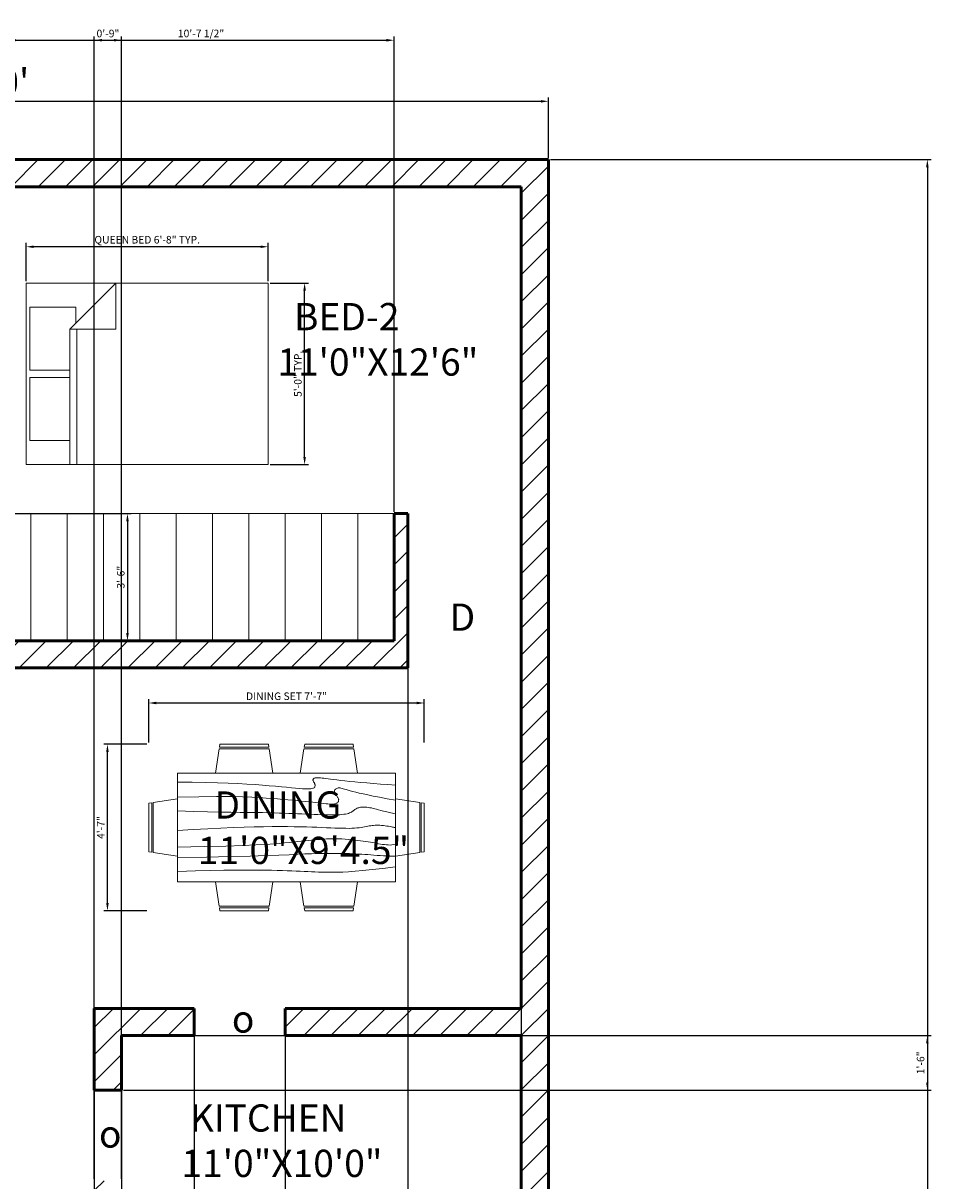
# Model space of a CAD drawing. Units: inches. Extents: x 2758 to 3288, y 1211 to 2050.
# Tile 4 of 4: x 2988 to 3288, y 1667 to 2050. Entities that reach past the tile are written whole.
import ezdxf

# ---------------------------------------------------------------- set-up
doc = ezdxf.new("R2010")
doc.units = ezdxf.units.IN
for name, color, linetype, lineweight in [('A-ANNO-DIMS', 2, 'Continuous', 18), ('A-AREA-IDEN', 7, 'Continuous', 25), ('A-FURN', 8, 'Continuous', 18), ('A-WALL', 7, 'Continuous', 50)]:
    doc.layers.add(name, color=color, linetype=linetype, lineweight=lineweight)
for name, color, linetype, lineweight, true_color in [('A-ANNO-TEXT', 244, 'Continuous', 18, 0x991b1e), ('A-FLOR-CASE', 244, 'Continuous', 18, 0x991b1e), ('A-WALL-PATT', 244, 'Continuous', 13, 0x991b1e)]:
    doc.layers.add(name, color=color, linetype=linetype, lineweight=lineweight, true_color=true_color)
doc.styles.get("Standard").update_dxf_attribs({"font": 'arial.ttf'})
doc.dimstyles.new('ISO-25', dxfattribs={"dimtxt": 2.5, "dimasz": 2.5, "dimexe": 1.25, "dimexo": 0.625, "dimtad": 1, "dimlunit": 3, "dimtxsty": 'Standard', "dimcen": 2.5, "dimadec": 0, "dimazin": 0, "dimtfac": 1, "dimtmove": 0, "dimatfit": 3, "dimfxl": 1, "dimarcsym": 0})

# ---------------------------------------------------------------- blocks, each defined once
blk = doc.blocks.new('Dining Set - 36 x 72 in.')
for p, q in [((-22, 27.5), (-22.1562, 26.50042)), ((-22, 27.5), (-6, 27.5)), ((-5.8437, 26.49966), (-6, 27.5)), ((6, 27.5), (5.8438, 26.50042)), ((6, 27.5), (22, 27.5)), ((22.1563, 26.49966), (22, 27.5)), ((-22.2343, 26.00059), (-23.4847, 17.99762)), ((-22.2304, 26), (-5.7608, 26)), ((-5.8416, 26.5), (-22.1534, 26.5)), ((-4.5152, 17.99762), (-5.7655, 25.99926)), ((5.7657, 26.00059), (4.5153, 17.99762)), ((5.7696, 26), (22.2392, 26)), ((22.1584, 26.5), (5.8466, 26.5)), ((23.4848, 17.99762), (22.2345, 25.99926)), ((36, 18), (-36, 18)), ((-36, 18), (-36, -18)), ((36, -18), (36, 18)), ((-45.5, 8), (-44.5004, 8.15617)), ((-45.5, 8), (-45.5, -8)), ((-44.5, -8.15843), (-44.5, 8.15338)), ((-44.0006, 8.23428), (-35.9976, 9.48474)), ((-44, 8.23041), (-44, -8.23915)), ((44.0006, 8.23428), (35.9976, 9.48474)), ((44, 8.23041), (44, -8.23915)), ((44.5, -8.15843), (44.5, 8.15338)), ((45.5, 8), (44.5005, 8.15617)), ((45.5, 8), (45.5, -8)), ((-44.4997, -8.15631), (-45.5, -8)), ((-35.9976, -9.48476), (-43.9993, -8.2345)), ((35.9976, -9.48476), (43.9993, -8.2345)), ((44.4997, -8.15631), (45.5, -8)), ((-36, -18), (36, -18)), ((-22.2343, -26.0006), (-23.4847, -17.99762)), ((-4.5152, -17.99762), (-5.7655, -25.99928)), ((5.7657, -26.0006), (4.5153, -17.99762)), ((23.4848, -17.99762), (22.2345, -25.99928)), ((-22.2304, -26), (-5.7608, -26)), ((-22, -27.5), (-22.1562, -26.50044)), ((-5.8416, -26.5), (-22.1534, -26.5)), ((-5.8437, -26.49967), (-6, -27.5)), ((5.7696, -26), (22.2392, -26)), ((6, -27.5), (5.8438, -26.50044)), ((22.1584, -26.5), (5.8466, -26.5)), ((22.1563, -26.49967), (22, -27.5)), ((-22, -27.5), (-6, -27.5)), ((6, -27.5), (22, -27.5))]:
    blk.add_line(p, q)
for points in [[(-36, 15), (-31.1772, 14.97754), (-26.8079, 14.91406), (-22.8538, 14.81543), (-19.276, 14.6875), (-16.0362, 14.53613), (-13.0957, 14.36718), (-10.4159, 14.18652), (-7.9583, 14), (-5.6904, 13.81315), (-3.6035, 13.63021), (-1.6954, 13.45508), (0.0365, 13.29166), (1.5945, 13.14388), (2.9811, 13.01562), (4.1988, 12.9108), (5.25, 12.83333), (6.1393, 12.78613), (6.8802, 12.76823), (7.4883, 12.77767), (7.9792, 12.8125), (8.3685, 12.87077), (8.6719, 12.95052), (8.9049, 13.0498), (9.0833, 13.16666), (9.2205, 13.29899), (9.3216, 13.44401), (9.3895, 13.59879), (9.4271, 13.76041), (9.4373, 13.92594), (9.4232, 14.09245), (9.3875, 14.257), (9.3333, 14.41666), (9.2638, 14.56917), (9.1836, 14.71484), (9.0975, 14.85465), (9.0104, 14.98958), (8.9272, 15.1206), (8.8529, 15.2487), (8.7922, 15.37483), (8.75, 15.5), (8.7305, 15.62467), (8.7344, 15.74739), (8.7617, 15.86621), (8.8125, 15.97916), (8.8867, 16.08431), (8.9844, 16.17968), (9.1055, 16.26334), (9.25, 16.33333), (9.4189, 16.38802), (9.6172, 16.42708), (9.8506, 16.45052), (10.125, 16.45833), (10.4463, 16.45052), (10.8203, 16.42708), (11.2529, 16.38802), (11.75, 16.33333), (12.3184, 16.26318), (12.9694, 16.17838), (13.7151, 16.07991), (14.5677, 15.96875), (15.5395, 15.84586), (16.6426, 15.71224), (17.8893, 15.56884), (19.2917, 15.41666), (20.859, 15.25667), (22.5879, 15.08984), (24.4721, 14.91715), (26.5052, 14.73958), (28.6809, 14.5581), (30.9929, 14.3737), (33.4347, 14.18733), (36, 14)], [(-36, 10), (-28.9766, 10.14274), (-23.1725, 10.20442), (-18.4241, 10.19775), (-14.5677, 10.13541), (-11.4399, 10.03011), (-8.877, 9.89453), (-6.7154, 9.74137), (-4.7917, 9.58333), (-2.9698, 9.43082), (-1.2246, 9.28515), (0.4415, 9.14534), (2.026, 9.01041), (3.5266, 8.87939), (4.9408, 8.7513), (6.266, 8.62516), (7.5, 8.5), (8.6411, 8.37549), (9.6914, 8.2539), (10.6538, 8.13818), (11.5312, 8.03125), (12.3267, 7.93603), (13.043, 7.85547), (13.6831, 7.79248), (14.25, 7.75), (14.7471, 7.7303), (15.1797, 7.73307), (15.5537, 7.75732), (15.875, 7.80208), (16.1494, 7.86637), (16.3828, 7.94922), (16.5811, 8.04964), (16.75, 8.16666), (16.8944, 8.29915), (17.0143, 8.44531), (17.1089, 8.60319), (17.1771, 8.77083), (17.218, 8.94629), (17.2305, 9.1276), (17.2137, 9.31282), (17.1667, 9.5), (17.0895, 9.6875), (16.987, 9.875), (16.8649, 10.0625), (16.7292, 10.25), (16.5856, 10.4375), (16.4401, 10.625), (16.2985, 10.8125), (16.1667, 11), (16.05, 11.18733), (15.9518, 11.3737), (15.8752, 11.5581), (15.8229, 11.73958), (15.798, 11.91715), (15.8034, 12.08984), (15.842, 12.25667), (15.9167, 12.41666), (16.0295, 12.56836), (16.1784, 12.70833), (16.3605, 12.83268), (16.5729, 12.9375), (16.8127, 13.01888), (17.0768, 13.07291), (17.3625, 13.0957), (17.6667, 13.08333), (17.9894, 13.03312), (18.3418, 12.94726), (18.7382, 12.82918), (19.1927, 12.68229), (19.7195, 12.51001), (20.3327, 12.31575), (21.0465, 12.10294), (21.875, 11.875), (22.8357, 11.63354), (23.959, 11.37304), (25.2786, 11.08618), (26.8282, 10.76562), (28.6414, 10.40405), (30.752, 9.99414), (33.1936, 9.52856), (36, 9)], [(-36, 5.5), (-30.7157, 5.3348), (-26.069, 5.20963), (-21.9946, 5.11767), (-18.4271, 5.05208), (-15.3009, 5.00602), (-12.5508, 4.97265), (-10.1112, 4.94515), (-7.9167, 4.91666), (-5.909, 4.88167), (-4.0586, 4.83984), (-2.3429, 4.79215), (-0.7396, 4.73958), (0.7739, 4.6831), (2.22, 4.6237), (3.6213, 4.56233), (5, 4.5), (6.373, 4.43782), (7.7344, 4.3776), (9.0723, 4.32129), (10.375, 4.27083), (11.6309, 4.22819), (12.8281, 4.19531), (13.9551, 4.17415), (15, 4.16666), (15.954, 4.17448), (16.819, 4.19791), (17.6001, 4.23698), (18.3021, 4.29166), (18.9299, 4.36198), (19.4883, 4.44791), (19.9823, 4.54948), (20.4167, 4.66666), (20.7969, 4.79899), (21.1302, 4.94401), (21.4245, 5.09879), (21.6875, 5.26041), (21.9271, 5.42594), (22.1511, 5.59245), (22.3672, 5.757), (22.5834, 5.91666), (22.8065, 6.06868), (23.0404, 6.21093), (23.2879, 6.34147), (23.5521, 6.45833), (23.8358, 6.55957), (24.142, 6.64323), (24.4735, 6.70735), (24.8334, 6.75), (25.2235, 6.76969), (25.642, 6.76692), (26.0858, 6.74267), (26.5521, 6.69791), (27.0379, 6.63362), (27.5404, 6.55078), (28.0565, 6.45036), (28.5834, 6.33333), (29.1242, 6.19987), (29.7071, 6.04687), (30.3661, 5.87044), (31.1354, 5.66666), (32.0493, 5.43164), (33.142, 5.16146), (34.4475, 4.85221), (36, 4.5)], [(-36, -1), (-30.7915, -0.6591), (-26.0195, -0.38216), (-21.6519, -0.16284), (-17.6563, 0.00521), (-14.0005, 0.12833), (-10.6523, 0.21289), (-7.5796, 0.26522), (-4.75, 0.29166), (-2.134, 0.29793), (0.2878, 0.28711), (2.5317, 0.26163), (4.6146, 0.22396), (6.5529, 0.17651), (8.3633, 0.12174), (10.0623, 0.06209), (11.6667, 0), (13.1899, -0.06201), (14.6341, -0.1211), (15.9982, -0.17432), (17.2813, -0.21875), (18.4823, -0.25147), (19.6003, -0.26953), (20.6343, -0.27002), (21.5834, -0.25), (22.4481, -0.20768), (23.2357, -0.14584), (23.9549, -0.06836), (24.6146, 0.02083), (25.2235, 0.11784), (25.7904, 0.21875), (26.3241, 0.31966), (26.8334, 0.41666), (27.3265, 0.50618), (27.8099, 0.58593), (28.2894, 0.65397), (28.7709, 0.70833), (29.2601, 0.74707), (29.763, 0.76823), (30.2855, 0.76985), (30.8334, 0.75), (31.4088, 0.70784), (31.9994, 0.64713), (32.589, 0.57275), (33.1615, 0.48958), (33.7008, 0.4025), (34.1908, 0.3164), (34.6153, 0.23616), (34.9584, 0.16666), (35.2099, 0.11165), (35.3848, 0.07031), (35.504, 0.04069), (35.5886, 0.02083), (35.6594, 0.00879), (35.7377, 0.0026), (35.8442, 0.00032), (36, 0)], [(-36, -6.5), (-27.1843, -6.31267), (-20.084, -6.1263), (-14.469, -5.9419), (-10.1094, -5.76042), (-6.7752, -5.58285), (-4.2363, -5.41016), (-2.2629, -5.24333), (-0.625, -5.08334), (0.8708, -4.93099), (2.2715, -4.78646), (3.5872, -4.64974), (4.8281, -4.52084), (6.0046, -4.39974), (7.127, -4.28646), (8.2053, -4.18099), (9.25, -4.08334), (10.2705, -3.99382), (11.2734, -3.91407), (12.2647, -3.84603), (13.25, -3.79167), (14.2354, -3.75293), (15.2266, -3.73177), (16.2295, -3.73015), (17.25, -3.75), (18.2912, -3.79248), (19.3451, -3.85547), (20.4009, -3.93604), (21.4479, -4.03125), (22.4754, -4.13819), (23.4727, -4.25391), (24.4289, -4.37549), (25.3334, -4.5), (26.1785, -4.62492), (26.9694, -4.74935), (27.7145, -4.87281), (28.4219, -4.99479), (29.1, -5.11483), (29.7572, -5.23242), (30.4016, -5.34709), (31.0417, -5.45834), (31.6837, -5.56437), (32.3262, -5.65821), (32.9658, -5.73153), (33.599, -5.77604), (34.2224, -5.78345), (34.8327, -5.74545), (35.4264, -5.65373), (36, -5.5)], [(-36, -10), (-26.4022, -9.81299), (-18.4675, -9.62891), (-11.9839, -9.45069), (-6.7396, -9.28125), (-2.5226, -9.12354), (0.8789, -8.98047), (3.6769, -8.85498), (6.0833, -8.75), (8.2767, -8.66765), (10.3021, -8.60677), (12.1712, -8.56543), (13.8958, -8.54167), (15.4876, -8.53353), (16.9583, -8.53907), (18.3197, -8.55632), (19.5834, -8.58334), (20.7616, -8.61841), (21.8685, -8.66081), (22.9188, -8.71004), (23.9271, -8.76563), (24.9081, -8.82707), (25.8763, -8.89388), (26.8465, -8.96558), (27.8334, -9.04167), (28.8474, -9.12118), (29.8828, -9.20117), (30.93, -9.27824), (31.9792, -9.34896), (33.0205, -9.40991), (34.0443, -9.45768), (35.0407, -9.48885), (36, -9.5)], [(-36, -14.5), (-30.0881, -14.33513), (-25.0332, -14.21224), (-20.7312, -14.12647), (-17.0781, -14.07292), (-13.97, -14.04671), (-11.3027, -14.04297), (-8.9724, -14.05681), (-6.875, -14.08334), (-4.9224, -14.11833), (-3.0905, -14.16016), (-1.3709, -14.20785), (0.2448, -14.26042), (1.7647, -14.3169), (3.1973, -14.3763), (4.5507, -14.43767), (5.8333, -14.5), (7.0554, -14.5621), (8.235, -14.62175), (9.3922, -14.67652), (10.5469, -14.72396), (11.7192, -14.76164), (12.929, -14.78711), (14.1965, -14.79794), (15.5417, -14.79167), (16.9933, -14.76424), (18.6152, -14.70508), (20.4804, -14.60197), (22.6615, -14.44271), (25.2312, -14.21509), (28.2624, -13.9069), (31.8277, -13.50594), (36, -13)]]:
    blk.add_lwpolyline(points)
blk = doc.blocks.new('Bed - Queen')
for p, q in [((0, -80.00003), (0, 0)), ((0, 0), (59.99999, 0)), ((59.99999, 0), (59.99999, -80.00003)), ((7.99999, -1.2), (28.79998, -1.2)), ((7.99999, -14.4), (7.99999, -1.2)), ((28.79998, -1.2), (28.79998, -14.4)), ((31.19999, -1.2), (51.99999, -1.2)), ((31.19999, -14.4), (31.19999, -1.2)), ((51.99999, -1.2), (51.99999, -16.4)), ((0, -14.4), (44.8, -14.4)), ((59.99999, -29.6), (44.8, -14.4)), ((44.8, -14.4), (44.8, -29.6)), ((44.8, -16.8), (0, -16.8)), ((51.99999, -16.4), (46.79936, -16.4)), ((44.8, -29.6), (59.99999, -29.6)), ((59.99999, -80.00003), (0, -80.00003))]:
    blk.add_line(p, q)
blk = doc.blocks.new('*D6')
at = {"layer": 'A-ANNO-DIMS', "color": 0, "lineweight": -2, "transparency": 16777216}
for p, q in [((2801.14, 2005.44), (2801.14, 2025.32)), ((2803.64, 2024.07), (3158.64, 2024.07)), ((3161.14, 2005.44), (3161.14, 2025.32))]:
    blk.add_line(p, q, dxfattribs=at)
at = {"layer": 'A-ANNO-DIMS', "color": 0, "transparency": 16777216}
for points in [[(2803.64, 2024.49), (2803.64, 2023.65), (2801.14, 2024.07)], [(3158.64, 2024.49), (3158.64, 2023.65), (3161.14, 2024.07)]]:
    blk.add_solid(points, dxfattribs=at)
at = {"layer": 'Defpoints', "color": 0, "transparency": 16777216}
for p in [(3161.14, 2024.07), (2801.14, 2004.81), (3161.14, 2004.81)]:
    blk.add_point(p, dxfattribs=at)
at = {"layer": 'A-ANNO-DIMS', "color": 0, "transparency": 16777216, "insert": (2981.14, 2029.29), "char_height": 9, "attachment_point": 5}
blk.add_mtext("30'", dxfattribs=at)
blk = doc.blocks.new('*D8')
at = {"layer": 'A-ANNO-DIMS', "color": 0, "lineweight": -2, "transparency": 16777216}
for p, q in [((2988.6, 1964.64), (2988.6, 1977.26)), ((3066.1, 1976.01), (2991.1, 1976.01)), ((3068.6, 1964.64), (3068.6, 1977.26))]:
    blk.add_line(p, q, dxfattribs=at)
at = {"layer": 'A-ANNO-DIMS', "color": 0, "transparency": 16777216}
for points in [[(2991.1, 1976.43), (2991.1, 1975.6), (2988.6, 1976.01)], [(3066.1, 1976.43), (3066.1, 1975.6), (3068.6, 1976.01)]]:
    blk.add_solid(points, dxfattribs=at)
at = {"layer": 'Defpoints', "color": 0, "transparency": 16777216}
for p in [(2988.6, 1976.01), (2988.6, 1964.01), (3068.6, 1964.01)]:
    blk.add_point(p, dxfattribs=at)
at = {"layer": 'A-ANNO-DIMS', "color": 0, "transparency": 16777216, "insert": (3028.6, 1978.01), "char_height": 2.5, "attachment_point": 5}
blk.add_mtext('QUEEN BED 6\'-8" TYP.', dxfattribs=at)
blk = doc.blocks.new('*D9')
at = {"layer": 'A-ANNO-DIMS', "color": 0, "lineweight": -2, "transparency": 16777216}
for p, q in [((3069.23, 1964.01), (3081.85, 1964.01)), ((3080.6, 1906.51), (3080.6, 1961.51)), ((3069.23, 1904.01), (3081.85, 1904.01))]:
    blk.add_line(p, q, dxfattribs=at)
at = {"layer": 'A-ANNO-DIMS', "color": 0, "transparency": 16777216}
for points in [[(3080.18, 1961.51), (3081.02, 1961.51), (3080.6, 1964.01)], [(3080.18, 1906.51), (3081.02, 1906.51), (3080.6, 1904.01)]]:
    blk.add_solid(points, dxfattribs=at)
at = {"layer": 'Defpoints', "color": 0, "transparency": 16777216}
for p in [(3068.6, 1964.01), (3080.6, 1964.01), (3068.6, 1904.01)]:
    blk.add_point(p, dxfattribs=at)
at = {"layer": 'A-ANNO-DIMS', "color": 0, "transparency": 16777216, "insert": (3078.7, 1934.01), "char_height": 2.5, "attachment_point": 5, "rotation": 90}
blk.add_mtext('5\'-0" TYP.', dxfattribs=at)
blk = doc.blocks.new('*D12')
at = {"layer": 'A-ANNO-DIMS', "color": 0, "lineweight": -2, "transparency": 16777216}
for p, q in [((3029.13, 1812.2), (3029.13, 1826.48)), ((3031.63, 1825.23), (3117.63, 1825.23)), ((3120.13, 1812.2), (3120.13, 1826.48))]:
    blk.add_line(p, q, dxfattribs=at)
at = {"layer": 'A-ANNO-DIMS', "color": 0, "transparency": 16777216}
for points in [[(3031.63, 1825.65), (3031.63, 1824.81), (3029.13, 1825.23)], [(3117.63, 1825.65), (3117.63, 1824.81), (3120.13, 1825.23)]]:
    blk.add_solid(points, dxfattribs=at)
at = {"layer": 'Defpoints', "color": 0, "transparency": 16777216}
for p in [(3120.13, 1825.23), (3029.13, 1811.58), (3120.13, 1811.58)]:
    blk.add_point(p, dxfattribs=at)
at = {"layer": 'A-ANNO-DIMS', "color": 0, "transparency": 16777216, "insert": (3074.63, 1827.15), "char_height": 2.5, "attachment_point": 5}
blk.add_mtext('DINING SET 7\'-7"', dxfattribs=at)
blk = doc.blocks.new('*D13')
at = {"layer": 'A-ANNO-DIMS', "color": 0, "lineweight": -2, "transparency": 16777216}
for p, q in [((3028.5, 1811.58), (3014.23, 1811.58)), ((3015.48, 1759.08), (3015.48, 1809.08)), ((3028.5, 1756.58), (3014.23, 1756.58))]:
    blk.add_line(p, q, dxfattribs=at)
at = {"layer": 'A-ANNO-DIMS', "color": 0, "transparency": 16777216}
for points in [[(3015.06, 1809.08), (3015.89, 1809.08), (3015.48, 1811.58)], [(3015.06, 1759.08), (3015.89, 1759.08), (3015.48, 1756.58)]]:
    blk.add_solid(points, dxfattribs=at)
at = {"layer": 'Defpoints', "color": 0, "transparency": 16777216}
for p in [(3015.48, 1811.58), (3029.13, 1811.58), (3029.13, 1756.58)]:
    blk.add_point(p, dxfattribs=at)
at = {"layer": 'A-ANNO-DIMS', "color": 0, "transparency": 16777216, "insert": (3013.6, 1784.08), "char_height": 2.5, "attachment_point": 5, "rotation": 90}
blk.add_mtext('4\'-7"', dxfattribs=at)
blk = doc.blocks.new('*D19')
at = {"layer": 'A-ANNO-DIMS', "color": 0, "lineweight": -2, "transparency": 16777216}
for p, q in [((3161.76, 2004.81), (3287.54, 2004.81)), ((3286.29, 2002.31), (3286.29, 1254.6)), ((3247.46, 1252.1), (3287.54, 1252.1))]:
    blk.add_line(p, q, dxfattribs=at)
at = {"layer": 'A-ANNO-DIMS', "color": 0, "transparency": 16777216}
for points in [[(3285.87, 2002.31), (3286.7, 2002.31), (3286.29, 2004.81)], [(3285.87, 1254.6), (3286.7, 1254.6), (3286.29, 1252.1)]]:
    blk.add_solid(points, dxfattribs=at)
at = {"layer": 'Defpoints', "color": 0, "transparency": 16777216}
for p in [(3161.14, 2004.81), (3246.84, 1252.1), (3286.29, 1252.1)]:
    blk.add_point(p, dxfattribs=at)
at = {"layer": 'A-ANNO-DIMS', "color": 0, "transparency": 16777216, "insert": (3284.37, 1628.45), "char_height": 2.5, "attachment_point": 5, "rotation": 90}
blk.add_mtext('62\'-8 1/2"', dxfattribs=at)
blk = doc.blocks.new('*D22')
at = {"layer": 'A-ANNO-DIMS', "color": 0, "lineweight": -2, "transparency": 16777216}
for p, q in [((3011.14, 1667.94), (3011.14, 2045.51)), ((3013.64, 2044.26), (3017.64, 2044.26)), ((3020.14, 1667.94), (3020.14, 2045.51))]:
    blk.add_line(p, q, dxfattribs=at)
at = {"layer": 'A-ANNO-DIMS', "color": 0, "transparency": 16777216}
for points in [[(3013.64, 2044.68), (3013.64, 2043.84), (3011.14, 2044.26)], [(3017.64, 2044.68), (3017.64, 2043.84), (3020.14, 2044.26)]]:
    blk.add_solid(points, dxfattribs=at)
at = {"layer": 'Defpoints', "color": 0, "transparency": 16777216}
for p in [(3020.14, 2044.26), (3011.14, 1667.31), (3020.14, 1667.31)]:
    blk.add_point(p, dxfattribs=at)
at = {"layer": 'A-ANNO-DIMS', "color": 0, "transparency": 16777216, "insert": (3015.64, 2046.16), "char_height": 2.5, "attachment_point": 5}
blk.add_mtext('0\'-9"', dxfattribs=at)
blk = doc.blocks.new('*D25')
at = {"layer": 'A-ANNO-DIMS', "color": 0, "lineweight": -2, "transparency": 16777216}
for p, q in [((3152.14, 1995.19), (3152.14, 1211.4)), ((3114.64, 1887.19), (3114.64, 1211.4)), ((3117.14, 1212.65), (3149.64, 1212.65))]:
    blk.add_line(p, q, dxfattribs=at)
at = {"layer": 'A-ANNO-DIMS', "color": 0, "transparency": 16777216}
for points in [[(3117.14, 1213.06), (3117.14, 1212.23), (3114.64, 1212.65)], [(3149.64, 1213.06), (3149.64, 1212.23), (3152.14, 1212.65)]]:
    blk.add_solid(points, dxfattribs=at)
at = {"layer": 'Defpoints', "color": 0, "transparency": 16777216}
for p in [(3152.14, 1995.81), (3114.64, 1887.81), (3152.14, 1212.65)]:
    blk.add_point(p, dxfattribs=at)
at = {"layer": 'A-ANNO-DIMS', "color": 0, "transparency": 16777216, "insert": (3133.39, 1214.57), "char_height": 2.5, "attachment_point": 5}
blk.add_mtext('3\'-1 1/2"', dxfattribs=at)
blk = doc.blocks.new('*D27')
at = {"layer": 'A-ANNO-DIMS', "color": 0, "lineweight": -2, "transparency": 16777216}
for p, q in [((3044.14, 1723.69), (3044.14, 1211.4)), ((3074.14, 1723.69), (3074.14, 1211.4)), ((3046.64, 1212.65), (3071.64, 1212.65))]:
    blk.add_line(p, q, dxfattribs=at)
at = {"layer": 'A-ANNO-DIMS', "color": 0, "transparency": 16777216}
for points in [[(3046.64, 1213.06), (3046.64, 1212.23), (3044.14, 1212.65)], [(3071.64, 1213.06), (3071.64, 1212.23), (3074.14, 1212.65)]]:
    blk.add_solid(points, dxfattribs=at)
at = {"layer": 'Defpoints', "color": 0, "transparency": 16777216}
for p in [(3044.14, 1724.31), (3074.14, 1724.31), (3074.14, 1212.65)]:
    blk.add_point(p, dxfattribs=at)
at = {"layer": 'A-ANNO-DIMS', "color": 0, "transparency": 16777216, "insert": (3059.14, 1214.55), "char_height": 2.5, "attachment_point": 5}
blk.add_mtext('2\'-6"', dxfattribs=at)
blk = doc.blocks.new('*D28')
at = {"layer": 'A-ANNO-DIMS', "color": 0, "lineweight": -2, "transparency": 16777216}
for p, q in [((2939.69, 1723.69), (2939.69, 1211.4)), ((3011.14, 1723.69), (3011.14, 1211.4)), ((2942.19, 1212.65), (3008.64, 1212.65))]:
    blk.add_line(p, q, dxfattribs=at)
at = {"layer": 'A-ANNO-DIMS', "color": 0, "transparency": 16777216}
for points in [[(2942.19, 1213.06), (2942.19, 1212.23), (2939.69, 1212.65)], [(3008.64, 1213.06), (3008.64, 1212.23), (3011.14, 1212.65)]]:
    blk.add_solid(points, dxfattribs=at)
at = {"layer": 'Defpoints', "color": 0, "transparency": 16777216}
for p in [(2939.69, 1724.31), (3011.14, 1724.31), (3011.14, 1212.65)]:
    blk.add_point(p, dxfattribs=at)
at = {"layer": 'A-ANNO-DIMS', "color": 0, "transparency": 16777216, "insert": (2975.42, 1214.56), "char_height": 2.5, "attachment_point": 5}
blk.add_mtext('5\'-11 1/2"', dxfattribs=at)
blk = doc.blocks.new('*D33')
at = {"layer": 'A-ANNO-DIMS', "color": 0, "lineweight": -2, "transparency": 16777216}
for p, q in [((2983.26, 1887.81), (3023.34, 1887.81)), ((3022.09, 1885.31), (3022.09, 1848.31)), ((2983.26, 1845.81), (3023.34, 1845.81))]:
    blk.add_line(p, q, dxfattribs=at)
at = {"layer": 'A-ANNO-DIMS', "color": 0, "transparency": 16777216}
for points in [[(3021.67, 1885.31), (3022.51, 1885.31), (3022.09, 1887.81)], [(3021.67, 1848.31), (3022.51, 1848.31), (3022.09, 1845.81)]]:
    blk.add_solid(points, dxfattribs=at)
at = {"layer": 'Defpoints', "color": 0, "transparency": 16777216}
for p in [(2982.64, 1887.81), (2982.64, 1845.81), (3022.09, 1845.81)]:
    blk.add_point(p, dxfattribs=at)
at = {"layer": 'A-ANNO-DIMS', "color": 0, "transparency": 16777216, "insert": (3020.19, 1866.81), "char_height": 2.5, "attachment_point": 5, "rotation": 90}
blk.add_mtext('3\'-6"', dxfattribs=at)
blk = doc.blocks.new('*D34')
at = {"layer": 'A-ANNO-DIMS', "color": 0, "lineweight": -2, "transparency": 16777216}
for p, q in [((2982.64, 1888.44), (2982.64, 2045.51)), ((2985.14, 2044.26), (3107.64, 2044.26)), ((3110.14, 1888.44), (3110.14, 2045.51))]:
    blk.add_line(p, q, dxfattribs=at)
at = {"layer": 'A-ANNO-DIMS', "color": 0, "transparency": 16777216}
for points in [[(2985.14, 2044.68), (2985.14, 2043.84), (2982.64, 2044.26)], [(3107.64, 2044.68), (3107.64, 2043.84), (3110.14, 2044.26)]]:
    blk.add_solid(points, dxfattribs=at)
at = {"layer": 'Defpoints', "color": 0, "transparency": 16777216}
for p in [(3110.14, 2044.26), (2982.64, 1887.81), (3110.14, 1887.81)]:
    blk.add_point(p, dxfattribs=at)
at = {"layer": 'A-ANNO-DIMS', "color": 0, "transparency": 16777216, "insert": (3046.39, 2046.18), "char_height": 2.5, "attachment_point": 5}
blk.add_mtext('10\'-7 1/2"', dxfattribs=at)
blk = doc.blocks.new('*D37')
at = {"layer": 'A-ANNO-DIMS', "color": 0, "lineweight": -2, "transparency": 16777216}
for p, q in [((3020.14, 1714.69), (3020.14, 1211.4)), ((3044.14, 1714.69), (3044.14, 1211.4)), ((3022.64, 1212.65), (3041.64, 1212.65))]:
    blk.add_line(p, q, dxfattribs=at)
at = {"layer": 'A-ANNO-DIMS', "color": 0, "transparency": 16777216}
for points in [[(3022.64, 1213.06), (3022.64, 1212.23), (3020.14, 1212.65)], [(3041.64, 1213.06), (3041.64, 1212.23), (3044.14, 1212.65)]]:
    blk.add_solid(points, dxfattribs=at)
at = {"layer": 'Defpoints', "color": 0, "transparency": 16777216}
for p in [(3020.14, 1715.31), (3044.14, 1715.31), (3044.14, 1212.65)]:
    blk.add_point(p, dxfattribs=at)
at = {"layer": 'A-ANNO-DIMS', "color": 0, "transparency": 16777216, "insert": (3032.14, 1214.55), "char_height": 2.5, "attachment_point": 5}
blk.add_mtext('2\'-0"', dxfattribs=at)
blk = doc.blocks.new('*D38')
at = {"layer": 'A-ANNO-DIMS', "color": 0, "lineweight": -2, "transparency": 16777216}
for p, q in [((3020.76, 1715.31), (3287.54, 1715.31)), ((3286.29, 1712.81), (3286.29, 1699.81)), ((3020.76, 1697.31), (3287.54, 1697.31))]:
    blk.add_line(p, q, dxfattribs=at)
at = {"layer": 'A-ANNO-DIMS', "color": 0, "transparency": 16777216}
for points in [[(3285.87, 1712.81), (3286.7, 1712.81), (3286.29, 1715.31)], [(3285.87, 1699.81), (3286.7, 1699.81), (3286.29, 1697.31)]]:
    blk.add_solid(points, dxfattribs=at)
at = {"layer": 'Defpoints', "color": 0, "transparency": 16777216}
for p in [(3020.14, 1715.31), (3020.14, 1697.31), (3286.29, 1697.31)]:
    blk.add_point(p, dxfattribs=at)
at = {"layer": 'A-ANNO-DIMS', "color": 0, "transparency": 16777216, "insert": (3284.38, 1706.31), "char_height": 2.5, "attachment_point": 5, "rotation": 90}
blk.add_mtext('1\'-6"', dxfattribs=at)

msp = doc.modelspace()

# ---------------------------------------------------------------- hatches: boundary and pattern name
at = {"layer": 'A-WALL-PATT'}
h = msp.add_hatch(dxfattribs=at)
h.set_pattern_fill('ANSI31', color=256, scale=2)
h.paths.add_polyline_path([(2810.139, 1377.81), (2810.139, 1715.31), (2939.691, 1715.31), (2939.691, 1724.31), (2910.639, 1724.31), (2910.639, 1778.31), (2906.139, 1778.31), (2906.139, 1724.31), (2896.389, 1724.31), (2810.139, 1724.31), (2810.139, 1796.31), (2982.639, 1796.31), (2982.639, 1800.81), (2810.139, 1800.81), (2810.139, 1920.81), (2872.139, 1920.81), (2872.139, 1929.81), (2810.139, 1929.81), (2810.139, 1995.81), (2890.139, 1995.81), (2890.139, 1920.81), (2973.639, 1920.81), (2973.639, 1841.31), (2949.639, 1841.31), (2949.639, 1836.81), (2973.639, 1836.81), (3114.639, 1836.81), (3114.639, 1887.81), (3110.139, 1887.81), (3110.139, 1845.81), (2982.639, 1845.81), (2982.639, 1977.81), (2973.639, 1977.81), (2973.639, 1929.81), (2894.639, 1929.81), (2894.639, 1995.81), (3152.139, 1995.81), (3152.139, 1800.81), (3152.139, 1796.31), (3152.139, 1724.31), (3074.139, 1724.31), (3074.139, 1715.31), (3152.139, 1715.31), (3152.139, 1595.31), (3020.139, 1595.31), (3020.139, 1667.31), (3011.139, 1667.31), (3011.139, 1586.31), (3080.139, 1586.31), (3080.139, 1284.81), (3089.139, 1284.81), (3089.139, 1586.31), (3161.139, 1586.31), (3161.139, 2004.81), (2801.139, 2004.81), (2801.139, 1284.81), (3032.139, 1284.81), (3032.139, 1320.81), (3023.139, 1320.81), (3023.139, 1293.81), (2810.139, 1293.81), (2810.139, 1368.81), (3032.139, 1368.81), (3032.139, 1377.81)])
h = msp.add_hatch(dxfattribs=at)
h.set_pattern_fill('ANSI31', color=256, scale=2)
h.paths.add_polyline_path([(3044.139, 1724.31), (3011.139, 1724.31), (3011.139, 1697.31), (3020.139, 1697.31), (3020.139, 1715.31), (3032.139, 1715.31), (3044.139, 1715.31)])

# ---------------------------------------------------------------- linework, layer by layer
at = {"layer": 'A-FLOR-CASE'}
for p, q in [((2982.639, 1887.81), (3114.639, 1887.81)), ((2990.139, 1845.81), (2990.139, 1887.81)), ((3002.139, 1845.81), (3002.139, 1887.81)), ((3014.139, 1845.81), (3014.139, 1887.81)), ((3026.139, 1845.81), (3026.139, 1887.81)), ((3038.139, 1845.81), (3038.139, 1887.81)), ((3050.139, 1845.81), (3050.139, 1887.81)), ((3062.139, 1845.81), (3062.139, 1887.81)), ((3074.139, 1845.81), (3074.139, 1887.81)), ((3086.139, 1845.81), (3086.139, 1887.81)), ((3098.139, 1845.81), (3098.139, 1887.81))]:
    msp.add_line(p, q, dxfattribs=at)
at = {"layer": 'A-WALL'}
for p, q in [((2801.139, 2004.81), (3161.139, 2004.81)), ((3161.139, 2004.81), (3161.139, 1586.31)), ((2894.639, 1995.81), (3152.139, 1995.81)), ((3152.139, 1995.81), (3152.139, 1800.81)), ((3110.139, 1887.81), (3114.639, 1887.81)), ((3110.139, 1845.81), (3110.139, 1887.81)), ((3114.639, 1887.81), (3114.639, 1836.81)), ((2982.639, 1845.81), (3110.139, 1845.81)), ((2973.639, 1836.81), (3114.639, 1836.81)), ((3152.139, 1796.31), (3152.139, 1800.81)), ((3152.139, 1796.31), (3152.139, 1724.31)), ((3011.139, 1724.31), (3011.139, 1697.31)), ((3011.139, 1724.31), (3044.139, 1724.31)), ((3044.139, 1715.31), (3044.139, 1724.31)), ((3074.139, 1715.31), (3074.139, 1724.31)), ((3074.139, 1724.31), (3152.139, 1724.31)), ((3020.139, 1715.31), (3020.139, 1697.31)), ((3020.139, 1715.31), (3044.139, 1715.31)), ((3020.139, 1715.31), (3032.139, 1715.31)), ((3032.139, 1715.31), (3044.139, 1715.31)), ((3074.139, 1715.31), (3152.139, 1715.31)), ((3152.139, 1715.31), (3152.139, 1595.31)), ((3011.139, 1697.31), (3020.139, 1697.31))]:
    msp.add_line(p, q, dxfattribs=at)

# ---------------------------------------------------------------- block references
at = {"layer": 'A-FURN', "rotation": 90}
msp.add_blockref('Bed - Queen', (2988.601, 1904.012), dxfattribs=at)
at = {"layer": 'A-FURN'}
msp.add_blockref('Dining Set - 36 x 72 in.', (3074.625, 1784.079), dxfattribs=at)

# ---------------------------------------------------------------- texts
at = {"layer": 'A-ANNO-TEXT', "char_height": 9, "attachment_point": 1}
for s, width, heights, insert in [('D', 25.77074, [19.217], (3128.488, 1858.094)), ('o', 14.11125, [10.571], (3056.565, 1725.288)), ('o', 25.45254, [19.689], (3012.675, 1687.299))]:
    msp.add_mtext_dynamic_manual_height_columns(s, width=width, gutter_width=12.5, heights=heights, dxfattribs=dict(at, insert=insert))
at = {"layer": 'A-AREA-IDEN', "char_height": 9, "attachment_point": 1}
for s, insert in [('  BED-2\\P11\'0"X12\'6"', (3071.591, 1957.415)), ('  DINING\\P11\'0"X9\'4.5"', (3045.32, 1796.02)), (' KITCHEN\\P11\'0"X10\'0"', (3039.915, 1692.581))]:
    msp.add_mtext_dynamic_manual_height_columns(s, width=130.32194, gutter_width=12.5, heights=[77.844], dxfattribs=dict(at, insert=insert))

# ---------------------------------------------------------------- dimensions: what is measured, and where the dimension line sits
at = {"layer": 'A-ANNO-DIMS'}
for base, p1, p2, override, picture, middle in [((3110.139, 2044.26), (2982.639, 1887.81), (3110.139, 1887.81), {"dimdec": 1, "dimlfac": 1, "dimrnd": 0, "dimzin": 1, "dimdsep": 46, "dimlunit": 4, "dimfrac": 2}, '*D34', (3046.389, 2046.178)), ((3020.139, 2044.26), (3011.139, 1667.31), (3020.139, 1667.31), {"dimdec": 1, "dimlfac": 1, "dimrnd": 0, "dimzin": 1, "dimdsep": 46, "dimlunit": 4, "dimfrac": 2}, '*D22', (3015.639, 2046.162)), ((3161.139, 2024.068), (2801.139, 2004.81), (3161.139, 2004.81), {"dimtxt": 9, "dimclrd": 0, "dimclre": 0, "dimclrt": 0}, '*D6', (2981.139, 2029.292)), ((3152.139, 1212.647), (3114.639, 1887.81), (3152.139, 1995.81), {"dimdec": 1, "dimlfac": 1, "dimrnd": 0, "dimzin": 1, "dimdsep": 46, "dimlunit": 4, "dimfrac": 2}, '*D25', (3133.389, 1214.566)), ((3011.139, 1212.647), (2939.691, 1724.31), (3011.139, 1724.31), {"dimdec": 1, "dimlfac": 1, "dimrnd": 0, "dimzin": 1, "dimdsep": 46, "dimlunit": 4, "dimfrac": 2}, '*D28', (2975.415, 1214.565)), ((3074.139, 1212.647), (3044.139, 1724.31), (3074.139, 1724.31), {"dimdec": 1, "dimlfac": 1, "dimrnd": 0, "dimzin": 1, "dimdsep": 46, "dimlunit": 4, "dimfrac": 2}, '*D27', (3059.139, 1214.549)), ((3044.139, 1212.647), (3020.139, 1715.31), (3044.139, 1715.31), {"dimdec": 1, "dimlfac": 1, "dimrnd": 0, "dimzin": 1, "dimdsep": 46, "dimlunit": 4, "dimfrac": 2}, '*D37', (3032.139, 1214.549))]:
    dim = msp.add_linear_dim(base=base, p1=p1, p2=p2, dimstyle='ISO-25', override=override, dxfattribs=at)
    dim.commit()
    dim.dimension.update_dxf_attribs({"geometry": picture, "text_midpoint": middle})
for base, p1, p2, angle, picture, middle in [((3286.286, 1252.097), (3161.139, 2004.81), (3246.836, 1252.097), 90, '*D19', (3284.368, 1628.454)), ((3022.089, 1845.81), (2982.639, 1887.81), (2982.639, 1845.81), 270, '*D33', (3020.187, 1866.81)), ((3015.475, 1811.579), (3029.125, 1756.579), (3029.125, 1811.579), 90, '*D13', (3013.6, 1784.079)), ((3286.286, 1697.31), (3020.139, 1715.31), (3020.139, 1697.31), 90, '*D38', (3284.384, 1706.31))]:
    dim = msp.add_linear_dim(base=base, p1=p1, p2=p2, angle=angle, dimstyle='ISO-25', override={"dimdec": 1, "dimlfac": 1, "dimrnd": 0, "dimzin": 1, "dimdsep": 46, "dimlunit": 4, "dimfrac": 2}, dxfattribs=at)
    dim.commit()
    dim.dimension.update_dxf_attribs({"geometry": picture, "text_midpoint": middle})
for base, p1, p2, angle, text, picture, middle in [((2988.601, 1976.012), (3068.601, 1964.012), (2988.601, 1964.012), 180, 'QUEEN BED <> TYP.', '*D8', (3028.601, 1978.007)), ((3080.601, 1964.012), (3068.601, 1904.012), (3068.601, 1964.012), 90, '<> TYP.', '*D9', (3078.699, 1934.012))]:
    dim = msp.add_linear_dim(base=base, p1=p1, p2=p2, angle=angle, text=text, dimstyle='ISO-25', override={"dimdec": 1, "dimlfac": 1, "dimrnd": 0, "dimzin": 1, "dimdsep": 46, "dimlunit": 4, "dimfrac": 2}, dxfattribs=at)
    dim.commit()
    dim.dimension.update_dxf_attribs({"geometry": picture, "text_midpoint": middle})
dim = msp.add_linear_dim(base=(3120.125, 1825.229), p1=(3029.125, 1811.579), p2=(3120.125, 1811.579), text='DINING SET <>', dimstyle='ISO-25', override={"dimdec": 1, "dimlfac": 1, "dimrnd": 0, "dimzin": 1, "dimdsep": 46, "dimlunit": 4, "dimfrac": 2}, dxfattribs=at)
dim.commit()
dim.dimension.update_dxf_attribs({"geometry": '*D12', "text_midpoint": (3074.625, 1827.147)})

doc.saveas('drawing.dxf')
